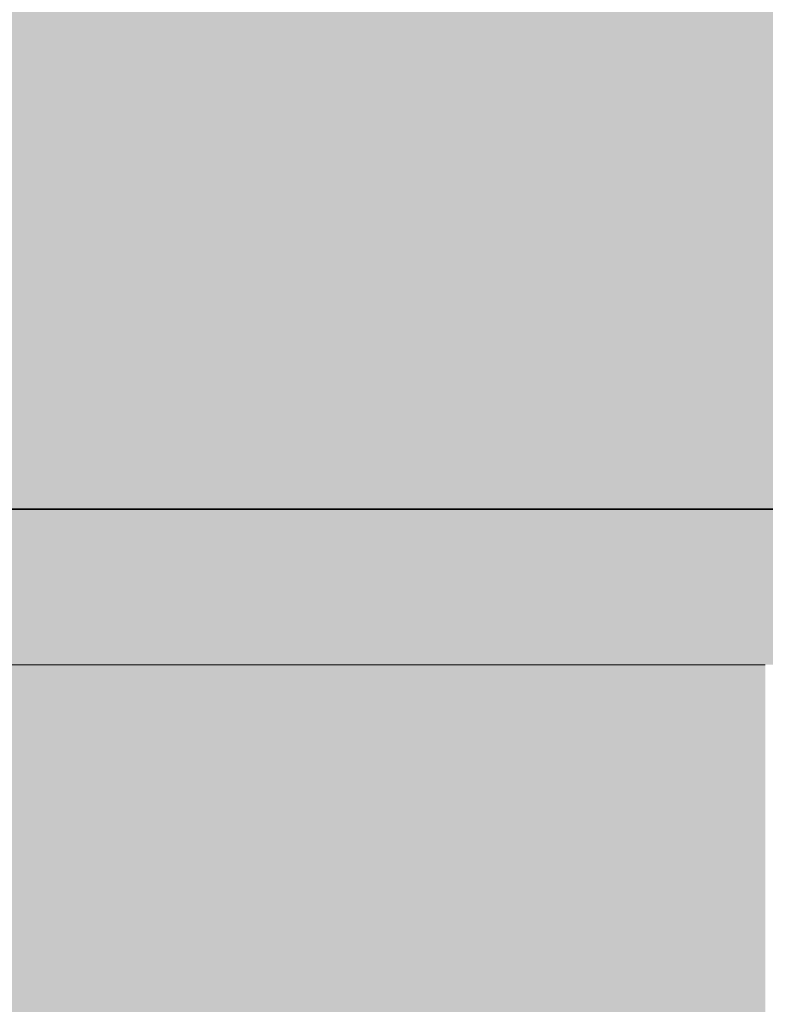
# Model space of a CAD drawing. Units: inches. Extents: x 1704 to 6393, y -157 to 1172.
# Tile 57 of 122: x 1931 to 1969, y 870 to 920. Entities that reach past the tile are written whole.
import ezdxf

# ---------------------------------------------------------------- set-up
doc = ezdxf.new("R2010")
doc.units = ezdxf.units.IN
doc.header["$MEASUREMENT"] = 0
for name, color, linetype, lineweight in [('A-ANNO-DIMS', 7, 'Continuous', 13), ('L-HRDS', 8, 'Continuous', 18), ('WALLS', 7, 'Continuous', 35)]:
    doc.layers.add(name, color=color, linetype=linetype, lineweight=lineweight)
doc.layers.add('L-HRDS-PATT', color=9, linetype='Continuous', lineweight=13, true_color=0xc5c1ba)
doc.layers.add('L-WATR-PATT', color=143, linetype='Continuous', lineweight=13, true_color=0x7ab0df)
doc.styles.get("Standard").update_dxf_attribs({"font": 'arial.ttf'})
doc.dimstyles.get("Standard").update_dxf_attribs({"dimtxt": 6, "dimasz": 2, "dimexe": 0.18, "dimexo": 0.0625, "dimgap": 0.09, "dimtad": 0, "dimtih": 1, "dimtoh": 1, "dimdec": 1, "dimzin": 0, "dimdsep": 46, "dimlunit": 3, "dimtxsty": 'Standard', "dimblk": 'ARCHTICK', "dimcen": 0.09, "dimadec": 0, "dimazin": 0, "dimtfac": 1, "dimtdec": 1, "dimtofl": 0, "dimtmove": 0, "dimatfit": 3, "dimfxl": 1, "dimtolj": 1, "dimtzin": 0, "dimarcsym": 0})

# ---------------------------------------------------------------- blocks, each defined once
blk = doc.blocks.new('_ArchTick')
at = {"color": 0, "linetype": 'ByBlock', "const_width": 0.15}
blk.add_lwpolyline([(-0.5, -0.5), (0.5, 0.5)], dxfattribs=at)
blk = doc.blocks.new('*D93')
at = {"layer": 'A-ANNO-DIMS', "color": 0, "lineweight": -2, "transparency": 16777216}
for p, q in [((2605.286, 895.213), (1829.698, 895.213)), ((1829.878, 895.213), (1829.878, 495.866)), ((1829.878, 90.213), (1829.878, 489.56)), ((2605.286, 90.213), (1829.698, 90.213))]:
    blk.add_line(p, q, dxfattribs=at)
at = {"layer": 'Defpoints', "color": 0, "lineweight": -3, "transparency": 16777216}
for p in [(2605.349, 895.213), (1829.878, 90.213), (2605.349, 90.213)]:
    blk.add_point(p, dxfattribs=at)
at = {"layer": 'A-ANNO-DIMS', "color": 0, "lineweight": -2, "transparency": 16777216, "xscale": 2, "yscale": 2, "zscale": 2}
for p, rotation in [((1829.878, 895.213), 90), ((1829.878, 90.213), 270)]:
    blk.add_blockref('_ArchTick', p, dxfattribs=dict(at, rotation=rotation))
at = {"layer": 'A-ANNO-DIMS', "color": 0, "transparency": 16777216, "insert": (1829.878, 492.713), "char_height": 6, "attachment_point": 5}
blk.add_mtext('\\A1;805', dxfattribs=at)
blk = doc.blocks.new('*D94')
at = {"layer": 'A-ANNO-DIMS', "color": 0, "lineweight": -2, "transparency": 16777216}
for p, q in [((1898.349, 895.275), (1898.349, 1105.287)), ((1898.349, 1105.107), (1979.39, 1105.107)), ((2073.349, 1105.107), (1992.307, 1105.107)), ((2073.349, 895.275), (2073.349, 1105.287))]:
    blk.add_line(p, q, dxfattribs=at)
at = {"layer": 'Defpoints', "color": 0, "lineweight": -3, "transparency": 16777216}
for p in [(2073.349, 1105.107), (1898.349, 895.213), (2073.349, 895.213)]:
    blk.add_point(p, dxfattribs=at)
at = {"layer": 'A-ANNO-DIMS', "color": 0, "lineweight": -2, "transparency": 16777216, "xscale": 2, "yscale": 2, "zscale": 2, "rotation": 180}
blk.add_blockref('_ArchTick', (1898.349, 1105.107), dxfattribs=at)
at = {"layer": 'A-ANNO-DIMS', "color": 0, "lineweight": -2, "transparency": 16777216, "xscale": 2, "yscale": 2, "zscale": 2}
blk.add_blockref('_ArchTick', (2073.349, 1105.107), dxfattribs=at)
at = {"layer": 'A-ANNO-DIMS', "color": 0, "transparency": 16777216, "insert": (1985.849, 1105.107), "char_height": 6, "attachment_point": 5}
blk.add_mtext('\\A1;175', dxfattribs=at)

msp = doc.modelspace()

# ---------------------------------------------------------------- hatches: boundary and pattern name
at = {"layer": 'L-HRDS-PATT', "transparency": 33554643}
h = msp.add_hatch(color=256, dxfattribs=at)
h.dxf.hatch_style = 1
h.paths.add_polyline_path([(2065.589, 1033.213), (1898.349, 1033.213), (1898.349, 895.213), (2065.589, 895.213)])
h = msp.add_hatch(color=256, dxfattribs=at)
h.dxf.hatch_style = 1
h.paths.add_polyline_path([(2073.349, 719.213), (2021.151, 719.213), (2021.151, 711.213), (2073.349, 711.213)])
h.paths.add_polyline_path([(1977.349, 719.213), (1969.349, 719.213), (1898.349, 719.213), (1898.349, 711.213), (1977.349, 711.213)])
h.paths.add_polyline_path([(1977.349, 895.213), (1898.349, 895.213), (1898.349, 887.213), (1969.349, 887.213), (1977.349, 887.213)])
at = {"layer": 'L-WATR-PATT'}
h = msp.add_hatch(color=256, dxfattribs=at)
h.dxf.hatch_style = 1
h.paths.add_polyline_path([(1969.349, 887.213), (1902.349, 887.213), (1902.349, 719.213), (1969.349, 719.213)])

# ---------------------------------------------------------------- linework, layer by layer
at = {"layer": 'L-HRDS'}
msp.add_line((1969.349, 887.213), (1898.349, 887.213), dxfattribs=at)
at = {"layer": 'WALLS'}
msp.add_line((2167.349, 895.213), (1898.349, 895.213), dxfattribs=at)

# ---------------------------------------------------------------- dimensions: what is measured, and where the dimension line sits
at = {"layer": 'A-ANNO-DIMS'}
dim = msp.add_linear_dim(base=(2073.349, 1105.107), p1=(1898.349, 895.213), p2=(2073.349, 895.213), dimstyle='Standard', override={"dimdec": 0, "dimlfac": 1, "dimrnd": 0, "dimzin": 0, "dimdsep": 46, "dimlunit": 2}, dxfattribs=at)
dim.commit()
dim.dimension.update_dxf_attribs({"geometry": '*D94', "text_midpoint": (1985.849, 1105.107)})
dim = msp.add_linear_dim(base=(1829.878, 90.213), p1=(2605.349, 895.213), p2=(2605.349, 90.213), angle=90, dimstyle='Standard', override={"dimdec": 0, "dimlfac": 1, "dimrnd": 0, "dimzin": 0, "dimdsep": 46, "dimlunit": 2}, dxfattribs=at)
dim.commit()
dim.dimension.update_dxf_attribs({"geometry": '*D93', "text_midpoint": (1829.878, 492.713)})

doc.saveas('drawing.dxf')
